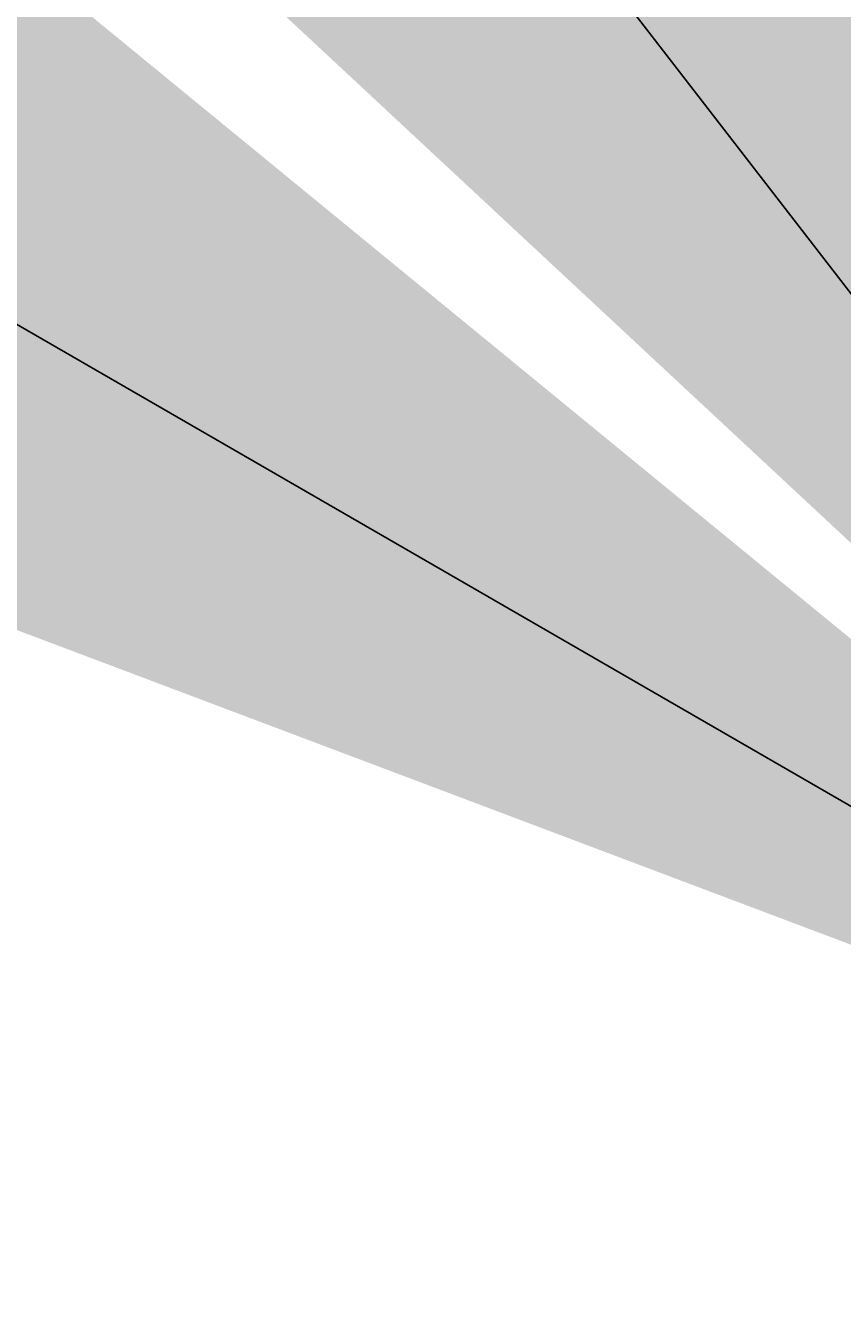
# Model space of a CAD drawing. Units: inches. Extents: x -9413 to 9703, y -9719 to 9096.
# Tile 1 of 1: x -5451 to -2479, y -311 to 4393. Entities that reach past the tile are written whole.
import ezdxf
from ezdxf import colors
from ezdxf.entities.mleader import LeaderData, LeaderLine
from ezdxf.math import Vec2, Vec3

# ---------------------------------------------------------------- set-up
doc = ezdxf.new("R2010")
doc.units = ezdxf.units.IN
doc.header["$MEASUREMENT"] = 0
doc.layers.add('M-ANNO-TEXT', color=7, linetype='Continuous', lineweight=18)
doc.styles.get("Standard").update_dxf_attribs({"font": 'arial.ttf'})

msp = doc.modelspace()

# ---------------------------------------------------------------- leaders
at = {"layer": 'M-ANNO-TEXT'}
ml = msp.add_multileader_mtext('Standard', dxfattribs=at)
ml.set_content('steam drum', color=256)
ml.set_leader_properties()
ml.build(insert=Vec2(0, 0))
ml.multileader.update_dxf_attribs({"dogleg_length": 0.36, "arrow_head_size": 10000, "scale": 10})
ctx = ml.context
ctx.base_point, ctx.scale, ctx.char_height, ctx.arrow_head_size, ctx.landing_gap_size, ctx.plane_origin = Vec3(1.078100315116472, 187.1657656808087), 10, 5.4, 10000, 0.9, Vec3(56.53630785249729, 178.1917761520126)
ctx.text_align_type = 2
notes = []
notes.append((ctx, [(0, (1, 1, 0), (49.60206616053652, 187.1657656808087), (-1, 0), 7.616326009130828, [(0, [(56.5363078524973, 178.1917761520126)], 0, [])])]))
ctx.mtext.insert, ctx.mtext.alignment, ctx.mtext.flow_direction = Vec3(41.08574015140569, 189.9099675907678), 3, 5
ml = msp.add_multileader_mtext('Standard', dxfattribs=at)
ml.set_content('Boiler', color=256)
ml.set_leader_properties()
ml.build(insert=Vec2(0, 0))
ml.multileader.update_dxf_attribs({"dogleg_length": 0.36, "arrow_head_size": 10000, "scale": 10})
ctx = ml.context
ctx.base_point, ctx.scale, ctx.char_height, ctx.arrow_head_size, ctx.landing_gap_size, ctx.plane_origin = Vec3(31.04430257849453, 103.0991380116177), 10, 5.4, 10000, 0.9, Vec3(69.11352005531556, 99.3051261342938)
ctx.text_align_type = 2
notes.append((ctx, [(0, (1, 1, 0), (62.54209871927075, 103.0991380116177), (-1, 0), 10.86041551321825, [(0, [(69.11352005531556, 99.3051261342938)], 0, [])])]))
ctx.mtext.insert, ctx.mtext.alignment, ctx.mtext.flow_direction = Vec3(50.7816832060525, 105.8433399215768), 3, 5
ml = msp.add_multileader_mtext('Standard', dxfattribs=at)
ml.set_content('Air preheater', color=256)
ml.set_leader_properties()
ml.build(insert=Vec2(0, 0))
ml.multileader.update_dxf_attribs({"dogleg_length": 0.36, "arrow_head_size": 10000, "scale": 10})
ctx = ml.context
ctx.base_point, ctx.scale, ctx.char_height, ctx.arrow_head_size, ctx.landing_gap_size, ctx.plane_origin = Vec3(229.7079293124727, 37.30650895205824), 10, 5.4, 10000, 0.9, Vec3(241.9833706008503, 78.04556948044049)
notes.append((ctx, [(1, (1, 1, 0), (223.7048975654645, 37.30650895205824), (1, 0), 6.003031747008185, [(0, [(241.9833706008503, 78.04556948044049)], 0, [])])]))
ctx.mtext.insert, ctx.mtext.flow_direction = Vec3(230.6079293124727, 40.75609967511417), 5
for ctx, leaders in notes:
    for number, flags, end, landing, length, lines in leaders:
        leader = LeaderData()
        leader.index, (leader.has_last_leader_line, leader.has_dogleg_vector, leader.attachment_direction) = number, flags
        leader.last_leader_point, leader.dogleg_vector, leader.dogleg_length = Vec3(end), Vec3(landing), length
        for number, points, colour, breaks in lines:
            line = LeaderLine()
            line.index, line.vertices, line.color, line.breaks = number, Vec3.list(points), colors.encode_raw_color(colour), breaks
            leader.lines.append(line)
        ctx.leaders.append(leader)

doc.saveas('drawing.dxf')
